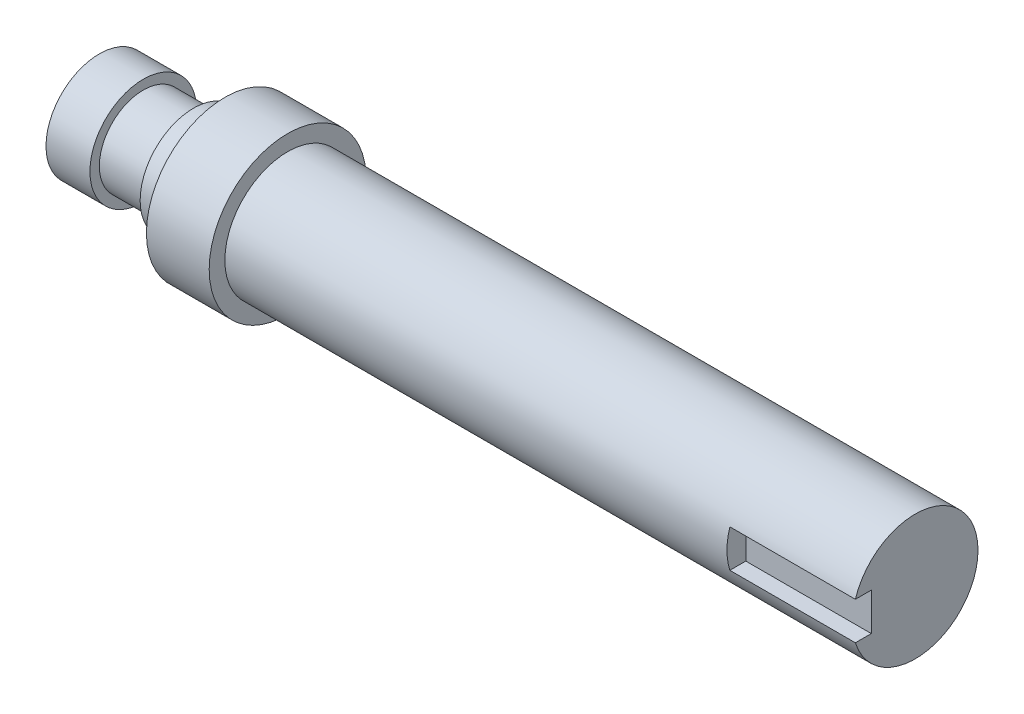
ISO-10303-21;
HEADER;
FILE_DESCRIPTION(('STEP AP214'),'2;1');
FILE_NAME('part.step','',(''),(''),'','','');
FILE_SCHEMA(('AUTOMOTIVE_DESIGN { 1 0 10303 214 1 1 1 1 }'));
ENDSEC;
DATA;
#1=APPLICATION_CONTEXT('core data for automotive mechanical design processes');
#2=APPLICATION_PROTOCOL_DEFINITION('international standard','automotive_design',2000,#1);
#3=PRODUCT_CONTEXT('',#1,'mechanical');
#4=PRODUCT('Part','Part','',(#3));
#5=PRODUCT_RELATED_PRODUCT_CATEGORY('part','',(#4));
#6=PRODUCT_DEFINITION_FORMATION('','',#4);
#7=PRODUCT_DEFINITION_CONTEXT('part definition',#1,'design');
#8=PRODUCT_DEFINITION('design','',#6,#7);
#9=PRODUCT_DEFINITION_SHAPE('','',#8);
#10=(LENGTH_UNIT() NAMED_UNIT(*) SI_UNIT(.MILLI.,.METRE.));
#11=(NAMED_UNIT(*) PLANE_ANGLE_UNIT() SI_UNIT($,.RADIAN.));
#12=(NAMED_UNIT(*) SI_UNIT($,.STERADIAN.) SOLID_ANGLE_UNIT());
#13=UNCERTAINTY_MEASURE_WITH_UNIT(LENGTH_MEASURE(1.E-05),#10,'distance_accuracy_value','');
#14=(GEOMETRIC_REPRESENTATION_CONTEXT(3) GLOBAL_UNCERTAINTY_ASSIGNED_CONTEXT((#13)) GLOBAL_UNIT_ASSIGNED_CONTEXT((#10,
#11,#12)) REPRESENTATION_CONTEXT('',''));
#15=CARTESIAN_POINT('',(0.,0.,0.));
#16=DIRECTION('',(0.,0.,1.));
#17=DIRECTION('',(1.,0.,0.));
#18=AXIS2_PLACEMENT_3D('',#15,#16,#17);
#19=CARTESIAN_POINT('',(0.,-8.5,0.));
#20=DIRECTION('',(-1.,0.,0.));
#21=DIRECTION('',(0.,0.,1.));
#22=AXIS2_PLACEMENT_3D('',#19,#20,#21);
#23=PLANE('',#22);
#24=CARTESIAN_POINT('',(0.,0.,0.));
#25=DIRECTION('',(-1.,0.,0.));
#26=DIRECTION('',(0.,0.,1.));
#27=AXIS2_PLACEMENT_3D('',#24,#25,#26);
#28=CIRCLE('',#27,8.5);
#29=CARTESIAN_POINT('',(0.,0.,8.5));
#30=VERTEX_POINT('',#29);
#31=EDGE_CURVE('E102',#30,#30,#28,.T.);
#32=ORIENTED_EDGE('',*,*,#31,.T.);
#33=EDGE_LOOP('',(#32));
#34=FACE_BOUND('',#33,.T.);
#35=ADVANCED_FACE('F41',(#34),#23,.T.);
#36=CARTESIAN_POINT('',(130.,0.,0.));
#37=DIRECTION('',(1.,0.,0.));
#38=DIRECTION('',(0.,0.,-1.));
#39=AXIS2_PLACEMENT_3D('',#36,#37,#38);
#40=PLANE('',#39);
#41=DIRECTION('',(0.,0.,1.));
#42=VECTOR('',#41,1.);
#43=CARTESIAN_POINT('',(130.,3.,7.));
#44=LINE('',#43,#42);
#45=CARTESIAN_POINT('',(130.,3.,7.));
#46=VERTEX_POINT('',#45);
#47=CARTESIAN_POINT('',(130.,3.,9.53939201416946));
#48=VERTEX_POINT('',#47);
#49=EDGE_CURVE('E104',#46,#48,#44,.T.);
#50=ORIENTED_EDGE('',*,*,#49,.F.);
#51=DIRECTION('',(0.,1.,0.));
#52=VECTOR('',#51,1.);
#53=CARTESIAN_POINT('',(130.,3.,7.));
#54=LINE('',#53,#52);
#55=CARTESIAN_POINT('',(130.,-3.,7.));
#56=VERTEX_POINT('',#55);
#57=EDGE_CURVE('E94',#56,#46,#54,.T.);
#58=ORIENTED_EDGE('',*,*,#57,.F.);
#59=DIRECTION('',(0.,0.,1.));
#60=VECTOR('',#59,1.);
#61=CARTESIAN_POINT('',(130.,-3.,7.));
#62=LINE('',#61,#60);
#63=CARTESIAN_POINT('',(130.,-3.,9.53939201416946));
#64=VERTEX_POINT('',#63);
#65=EDGE_CURVE('E84',#56,#64,#62,.T.);
#66=ORIENTED_EDGE('',*,*,#65,.T.);
#67=CARTESIAN_POINT('',(130.,0.,0.));
#68=DIRECTION('',(-1.,0.,0.));
#69=DIRECTION('',(0.,0.,1.));
#70=AXIS2_PLACEMENT_3D('',#67,#68,#69);
#71=CIRCLE('',#70,10.);
#72=EDGE_CURVE('E133',#48,#64,#71,.T.);
#73=ORIENTED_EDGE('',*,*,#72,.F.);
#74=EDGE_LOOP('',(#50,#58,#66,#73));
#75=FACE_BOUND('',#74,.T.);
#76=ADVANCED_FACE('F141',(#75),#40,.T.);
#77=CARTESIAN_POINT('',(0.,0.,0.));
#78=DIRECTION('',(-1.,0.,0.));
#79=DIRECTION('',(0.,0.,1.));
#80=AXIS2_PLACEMENT_3D('',#77,#78,#79);
#81=CYLINDRICAL_SURFACE('',#80,10.);
#82=DIRECTION('',(-1.,0.,0.));
#83=VECTOR('',#82,1.);
#84=CARTESIAN_POINT('',(0.,-3.,9.53939201416946));
#85=LINE('',#84,#83);
#86=CARTESIAN_POINT('',(110.,-3.,9.53939201416946));
#87=VERTEX_POINT('',#86);
#88=EDGE_CURVE('E11',#87,#64,#85,.F.);
#89=ORIENTED_EDGE('',*,*,#88,.F.);
#90=CARTESIAN_POINT('',(110.,0.,0.));
#91=DIRECTION('',(-1.,0.,0.));
#92=DIRECTION('',(0.,0.,1.));
#93=AXIS2_PLACEMENT_3D('',#90,#91,#92);
#94=CIRCLE('',#93,10.);
#95=CARTESIAN_POINT('',(110.,3.,9.53939201416946));
#96=VERTEX_POINT('',#95);
#97=EDGE_CURVE('E54',#96,#87,#94,.F.);
#98=ORIENTED_EDGE('',*,*,#97,.F.);
#99=DIRECTION('',(-1.,0.,0.));
#100=VECTOR('',#99,1.);
#101=CARTESIAN_POINT('',(0.,3.,9.53939201416946));
#102=LINE('',#101,#100);
#103=EDGE_CURVE('E48',#48,#96,#102,.T.);
#104=ORIENTED_EDGE('',*,*,#103,.F.);
#105=ORIENTED_EDGE('',*,*,#72,.T.);
#106=EDGE_LOOP('',(#89,#98,#104,#105));
#107=FACE_BOUND('',#106,.T.);
#108=CARTESIAN_POINT('',(30.,0.,0.));
#109=DIRECTION('',(-1.,0.,0.));
#110=DIRECTION('',(0.,0.,1.));
#111=AXIS2_PLACEMENT_3D('',#108,#109,#110);
#112=CIRCLE('',#111,10.);
#113=CARTESIAN_POINT('',(30.,0.,10.));
#114=VERTEX_POINT('',#113);
#115=EDGE_CURVE('E134',#114,#114,#112,.T.);
#116=ORIENTED_EDGE('',*,*,#115,.F.);
#117=EDGE_LOOP('',(#116));
#118=FACE_BOUND('',#117,.T.);
#119=ADVANCED_FACE('F139',(#107,#118),#81,.T.);
#120=CARTESIAN_POINT('',(30.,-10.,0.));
#121=DIRECTION('',(1.,0.,0.));
#122=DIRECTION('',(0.,0.,-1.));
#123=AXIS2_PLACEMENT_3D('',#120,#121,#122);
#124=PLANE('',#123);
#125=ORIENTED_EDGE('',*,*,#115,.T.);
#126=EDGE_LOOP('',(#125));
#127=FACE_BOUND('',#126,.T.);
#128=CARTESIAN_POINT('',(30.,0.,0.));
#129=DIRECTION('',(-1.,0.,0.));
#130=DIRECTION('',(0.,0.,1.));
#131=AXIS2_PLACEMENT_3D('',#128,#129,#130);
#132=CIRCLE('',#131,12.5);
#133=CARTESIAN_POINT('',(30.,0.,12.5));
#134=VERTEX_POINT('',#133);
#135=EDGE_CURVE('E126',#134,#134,#132,.T.);
#136=ORIENTED_EDGE('',*,*,#135,.F.);
#137=EDGE_LOOP('',(#136));
#138=FACE_BOUND('',#137,.T.);
#139=ADVANCED_FACE('F192',(#127,#138),#124,.T.);
#140=CARTESIAN_POINT('',(0.,0.,0.));
#141=DIRECTION('',(-1.,0.,0.));
#142=DIRECTION('',(0.,0.,1.));
#143=AXIS2_PLACEMENT_3D('',#140,#141,#142);
#144=CYLINDRICAL_SURFACE('',#143,12.5);
#145=ORIENTED_EDGE('',*,*,#135,.T.);
#146=EDGE_LOOP('',(#145));
#147=FACE_BOUND('',#146,.T.);
#148=CARTESIAN_POINT('',(20.,0.,0.));
#149=DIRECTION('',(-1.,0.,0.));
#150=DIRECTION('',(0.,0.,1.));
#151=AXIS2_PLACEMENT_3D('',#148,#149,#150);
#152=CIRCLE('',#151,12.5);
#153=CARTESIAN_POINT('',(20.,0.,12.5));
#154=VERTEX_POINT('',#153);
#155=EDGE_CURVE('E121',#154,#154,#152,.T.);
#156=ORIENTED_EDGE('',*,*,#155,.F.);
#157=EDGE_LOOP('',(#156));
#158=FACE_BOUND('',#157,.T.);
#159=ADVANCED_FACE('F186',(#147,#158),#144,.T.);
#160=CARTESIAN_POINT('',(20.,-12.5,0.));
#161=DIRECTION('',(-1.,0.,0.));
#162=DIRECTION('',(0.,0.,1.));
#163=AXIS2_PLACEMENT_3D('',#160,#161,#162);
#164=PLANE('',#163);
#165=ORIENTED_EDGE('',*,*,#155,.T.);
#166=EDGE_LOOP('',(#165));
#167=FACE_BOUND('',#166,.T.);
#168=CARTESIAN_POINT('',(20.,0.,0.));
#169=DIRECTION('',(-1.,0.,0.));
#170=DIRECTION('',(0.,0.,1.));
#171=AXIS2_PLACEMENT_3D('',#168,#169,#170);
#172=CIRCLE('',#171,8.5);
#173=CARTESIAN_POINT('',(20.,0.,8.5));
#174=VERTEX_POINT('',#173);
#175=EDGE_CURVE('E125',#174,#174,#172,.T.);
#176=ORIENTED_EDGE('',*,*,#175,.F.);
#177=EDGE_LOOP('',(#176));
#178=FACE_BOUND('',#177,.T.);
#179=ADVANCED_FACE('F181',(#167,#178),#164,.T.);
#180=CARTESIAN_POINT('',(0.,0.,0.));
#181=DIRECTION('',(-1.,0.,0.));
#182=DIRECTION('',(0.,0.,1.));
#183=AXIS2_PLACEMENT_3D('',#180,#181,#182);
#184=CYLINDRICAL_SURFACE('',#183,8.5);
#185=ORIENTED_EDGE('',*,*,#175,.T.);
#186=EDGE_LOOP('',(#185));
#187=FACE_BOUND('',#186,.T.);
#188=CARTESIAN_POINT('',(15.,0.,0.));
#189=DIRECTION('',(-1.,0.,0.));
#190=DIRECTION('',(0.,0.,1.));
#191=AXIS2_PLACEMENT_3D('',#188,#189,#190);
#192=CIRCLE('',#191,8.5);
#193=CARTESIAN_POINT('',(15.,0.,8.5));
#194=VERTEX_POINT('',#193);
#195=EDGE_CURVE('E118',#194,#194,#192,.T.);
#196=ORIENTED_EDGE('',*,*,#195,.F.);
#197=EDGE_LOOP('',(#196));
#198=FACE_BOUND('',#197,.T.);
#199=ADVANCED_FACE('F179',(#187,#198),#184,.T.);
#200=CARTESIAN_POINT('',(15.,-8.5,0.));
#201=DIRECTION('',(-1.,0.,0.));
#202=DIRECTION('',(0.,0.,1.));
#203=AXIS2_PLACEMENT_3D('',#200,#201,#202);
#204=PLANE('',#203);
#205=ORIENTED_EDGE('',*,*,#195,.T.);
#206=EDGE_LOOP('',(#205));
#207=FACE_BOUND('',#206,.T.);
#208=CARTESIAN_POINT('',(15.,0.,0.));
#209=DIRECTION('',(-1.,0.,0.));
#210=DIRECTION('',(0.,0.,1.));
#211=AXIS2_PLACEMENT_3D('',#208,#209,#210);
#212=CIRCLE('',#211,7.);
#213=CARTESIAN_POINT('',(15.,0.,7.));
#214=VERTEX_POINT('',#213);
#215=EDGE_CURVE('E119',#214,#214,#212,.T.);
#216=ORIENTED_EDGE('',*,*,#215,.F.);
#217=EDGE_LOOP('',(#216));
#218=FACE_BOUND('',#217,.T.);
#219=ADVANCED_FACE('F172',(#207,#218),#204,.T.);
#220=CARTESIAN_POINT('',(0.,0.,0.));
#221=DIRECTION('',(-1.,0.,0.));
#222=DIRECTION('',(0.,0.,1.));
#223=AXIS2_PLACEMENT_3D('',#220,#221,#222);
#224=CYLINDRICAL_SURFACE('',#223,7.);
#225=ORIENTED_EDGE('',*,*,#215,.T.);
#226=EDGE_LOOP('',(#225));
#227=FACE_BOUND('',#226,.T.);
#228=CARTESIAN_POINT('',(7.,0.,0.));
#229=DIRECTION('',(-1.,0.,0.));
#230=DIRECTION('',(0.,0.,1.));
#231=AXIS2_PLACEMENT_3D('',#228,#229,#230);
#232=CIRCLE('',#231,7.);
#233=CARTESIAN_POINT('',(7.,0.,7.));
#234=VERTEX_POINT('',#233);
#235=EDGE_CURVE('E114',#234,#234,#232,.T.);
#236=ORIENTED_EDGE('',*,*,#235,.F.);
#237=EDGE_LOOP('',(#236));
#238=FACE_BOUND('',#237,.T.);
#239=ADVANCED_FACE('F166',(#227,#238),#224,.T.);
#240=CARTESIAN_POINT('',(7.,-7.,0.));
#241=DIRECTION('',(1.,0.,0.));
#242=DIRECTION('',(0.,0.,-1.));
#243=AXIS2_PLACEMENT_3D('',#240,#241,#242);
#244=PLANE('',#243);
#245=ORIENTED_EDGE('',*,*,#235,.T.);
#246=EDGE_LOOP('',(#245));
#247=FACE_BOUND('',#246,.T.);
#248=CARTESIAN_POINT('',(7.,0.,0.));
#249=DIRECTION('',(-1.,0.,0.));
#250=DIRECTION('',(0.,0.,1.));
#251=AXIS2_PLACEMENT_3D('',#248,#249,#250);
#252=CIRCLE('',#251,8.5);
#253=CARTESIAN_POINT('',(7.,0.,8.5));
#254=VERTEX_POINT('',#253);
#255=EDGE_CURVE('E109',#254,#254,#252,.T.);
#256=ORIENTED_EDGE('',*,*,#255,.F.);
#257=EDGE_LOOP('',(#256));
#258=FACE_BOUND('',#257,.T.);
#259=ADVANCED_FACE('F162',(#247,#258),#244,.T.);
#260=CARTESIAN_POINT('',(0.,0.,0.));
#261=DIRECTION('',(-1.,0.,0.));
#262=DIRECTION('',(0.,0.,1.));
#263=AXIS2_PLACEMENT_3D('',#260,#261,#262);
#264=CYLINDRICAL_SURFACE('',#263,8.5);
#265=ORIENTED_EDGE('',*,*,#255,.T.);
#266=EDGE_LOOP('',(#265));
#267=FACE_BOUND('',#266,.T.);
#268=ORIENTED_EDGE('',*,*,#31,.F.);
#269=EDGE_LOOP('',(#268));
#270=FACE_BOUND('',#269,.T.);
#271=ADVANCED_FACE('F155',(#267,#270),#264,.T.);
#272=CARTESIAN_POINT('',(110.,0.,7.));
#273=DIRECTION('',(-1.,0.,0.));
#274=DIRECTION('',(0.,0.,1.));
#275=AXIS2_PLACEMENT_3D('',#272,#273,#274);
#276=PLANE('',#275);
#277=ORIENTED_EDGE('',*,*,#97,.T.);
#278=DIRECTION('',(0.,0.,1.));
#279=VECTOR('',#278,1.);
#280=CARTESIAN_POINT('',(110.,-3.,7.));
#281=LINE('',#280,#279);
#282=CARTESIAN_POINT('',(110.,-3.,7.));
#283=VERTEX_POINT('',#282);
#284=EDGE_CURVE('E76',#283,#87,#281,.T.);
#285=ORIENTED_EDGE('',*,*,#284,.F.);
#286=DIRECTION('',(0.,-1.,0.));
#287=VECTOR('',#286,1.);
#288=CARTESIAN_POINT('',(110.,-3.,7.));
#289=LINE('',#288,#287);
#290=CARTESIAN_POINT('',(110.,3.,7.));
#291=VERTEX_POINT('',#290);
#292=EDGE_CURVE('E82',#291,#283,#289,.T.);
#293=ORIENTED_EDGE('',*,*,#292,.F.);
#294=DIRECTION('',(0.,0.,1.));
#295=VECTOR('',#294,1.);
#296=CARTESIAN_POINT('',(110.,3.,7.));
#297=LINE('',#296,#295);
#298=EDGE_CURVE('E105',#291,#96,#297,.T.);
#299=ORIENTED_EDGE('',*,*,#298,.T.);
#300=EDGE_LOOP('',(#277,#285,#293,#299));
#301=FACE_BOUND('',#300,.T.);
#302=ADVANCED_FACE('F78',(#301),#276,.F.);
#303=CARTESIAN_POINT('',(110.,3.,7.));
#304=DIRECTION('',(0.,1.,0.));
#305=DIRECTION('',(0.,0.,1.));
#306=AXIS2_PLACEMENT_3D('',#303,#304,#305);
#307=PLANE('',#306);
#308=ORIENTED_EDGE('',*,*,#103,.T.);
#309=ORIENTED_EDGE('',*,*,#298,.F.);
#310=DIRECTION('',(-1.,0.,0.));
#311=VECTOR('',#310,1.);
#312=CARTESIAN_POINT('',(110.,3.,7.));
#313=LINE('',#312,#311);
#314=EDGE_CURVE('E81',#46,#291,#313,.T.);
#315=ORIENTED_EDGE('',*,*,#314,.F.);
#316=ORIENTED_EDGE('',*,*,#49,.T.);
#317=EDGE_LOOP('',(#308,#309,#315,#316));
#318=FACE_BOUND('',#317,.T.);
#319=ADVANCED_FACE('F145',(#318),#307,.F.);
#320=CARTESIAN_POINT('',(130.,-3.,7.));
#321=DIRECTION('',(0.,-1.,0.));
#322=DIRECTION('',(0.,0.,-1.));
#323=AXIS2_PLACEMENT_3D('',#320,#321,#322);
#324=PLANE('',#323);
#325=ORIENTED_EDGE('',*,*,#88,.T.);
#326=ORIENTED_EDGE('',*,*,#65,.F.);
#327=DIRECTION('',(1.,0.,0.));
#328=VECTOR('',#327,1.);
#329=CARTESIAN_POINT('',(130.,-3.,7.));
#330=LINE('',#329,#328);
#331=EDGE_CURVE('E86',#283,#56,#330,.T.);
#332=ORIENTED_EDGE('',*,*,#331,.F.);
#333=ORIENTED_EDGE('',*,*,#284,.T.);
#334=EDGE_LOOP('',(#325,#326,#332,#333));
#335=FACE_BOUND('',#334,.T.);
#336=ADVANCED_FACE('F90',(#335),#324,.F.);
#337=CARTESIAN_POINT('',(0.,0.,7.));
#338=DIRECTION('',(0.,0.,-1.));
#339=DIRECTION('',(-1.,0.,0.));
#340=AXIS2_PLACEMENT_3D('',#337,#338,#339);
#341=PLANE('',#340);
#342=ORIENTED_EDGE('',*,*,#292,.T.);
#343=ORIENTED_EDGE('',*,*,#331,.T.);
#344=ORIENTED_EDGE('',*,*,#57,.T.);
#345=ORIENTED_EDGE('',*,*,#314,.T.);
#346=EDGE_LOOP('',(#342,#343,#344,#345));
#347=FACE_BOUND('',#346,.T.);
#348=ADVANCED_FACE('F100',(#347),#341,.F.);
#349=CLOSED_SHELL('',(#35,#76,#119,#139,#159,#179,#199,#219,#239,#259,#271,#302,#319,#336,#348));
#350=MANIFOLD_SOLID_BREP('B2',#349);
#351=ADVANCED_BREP_SHAPE_REPRESENTATION('',(#18,#350),#14);
#352=SHAPE_DEFINITION_REPRESENTATION(#9,#351);
ENDSEC;
END-ISO-10303-21;
